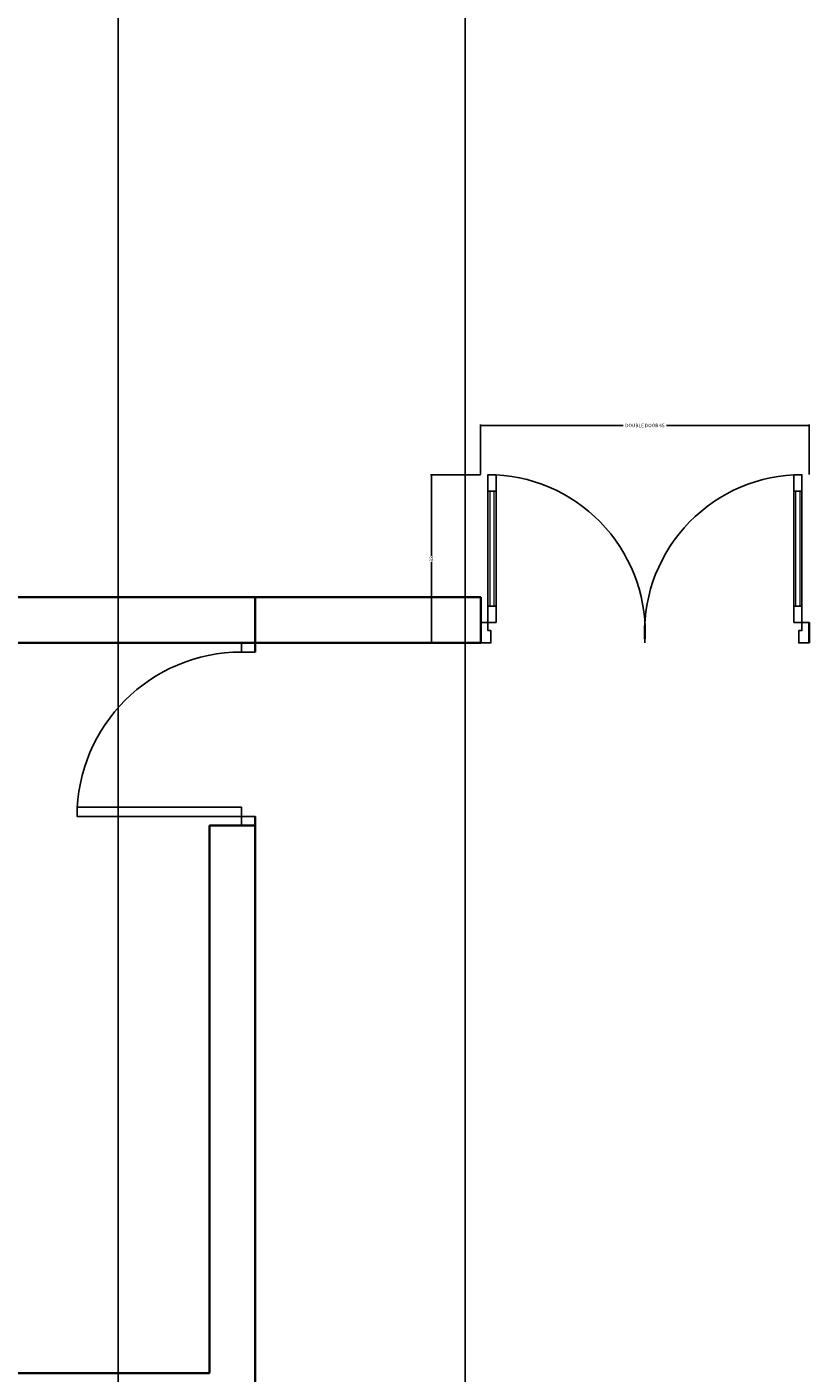
# Model space of a CAD drawing. Units: inches. Extents: x 867 to 1667, y -234 to 788.
# Tile 23 of 42: x 1212 to 1366, y -8 to 258. Entities that reach past the tile are written whole.
import ezdxf

# ---------------------------------------------------------------- set-up
doc = ezdxf.new("R2010")
doc.units = ezdxf.units.IN
doc.header["$MEASUREMENT"] = 0
for name, color, linetype, lineweight in [('A-ANNO-DIMS', 2, 'Continuous', 18), ('A-Door', 150, 'Continuous', 25), ('A-Glaz', 92, 'Continuous', 18), ('A-Wall', 7, 'Continuous', 35)]:
    doc.layers.add(name, color=color, linetype=linetype, lineweight=lineweight)
doc.layers.add('NET 01', color=8, linetype='Continuous')
doc.layers.add('NT', color=1, linetype='Continuous')
doc.styles.get("Standard").update_dxf_attribs({"font": 'arial.ttf'})
doc.dimstyles.get("Standard").update_dxf_attribs({"dimtxt": 0.6875, "dimasz": 0.18, "dimexe": 0.18, "dimexo": 0.0625, "dimgap": 0.09, "dimtad": 0, "dimdec": 4, "dimzin": 0, "dimdsep": 46, "dimlunit": 4, "dimtxsty": 'Standard', "dimcen": 0.09, "dimadec": 0, "dimazin": 0, "dimtfac": 1, "dimtdec": 4, "dimtofl": 0, "dimtmove": 0, "dimatfit": 3, "dimfxl": 1, "dimtolj": 1, "dimtzin": 0, "dimarcsym": 0})

# ---------------------------------------------------------------- blocks, each defined once
blk = doc.blocks.new('A$C292B336C')
at = {"layer": 'A-Door'}
for points in [[(-0.05, 0), (-0.05, 0.9), (0, 0.9), (0, 0)], [(-0.95, 0), (-0.95, -0.075), (-0.9, -0.075), (-0.9, 0)], [(0, 0), (0, -0.075), (0.05, -0.075), (0.05, 0)]]:
    blk.add_lwpolyline(points, close=True, dxfattribs=at)
at = {"layer": 'NET 01'}
blk.add_arc((0, 0), 0.9, 90, 180, dxfattribs=at)
blk = doc.blocks.new('A$C0EE93B68')
at = {"layer": 'A-Door'}
for points in [[(100, 1565), (100, 1600), (0, 1600), (0, 1550), (50, 1550), (60, 1550), (60, 1565)], [(100, 1525), (180, 1525), (180, 1565), (100, 1565)], [(180, 1525), (740, 1525), (740, 1565), (180, 1565)], [(820, 1525), (740, 1525), (740, 1565), (820, 1565)], [(100, 75), (180, 75), (180, 35), (100, 35)], [(180, 75), (740, 75), (740, 35), (180, 35)], [(820, 75), (740, 75), (740, 35), (820, 35)], [(100, 35), (100, 0), (0, 0), (0, 50), (50, 50), (60, 50), (60, 35)]]:
    blk.add_lwpolyline(points, close=True, dxfattribs=at)
at = {"layer": 'A-Glaz'}
for points in [[(180, 1535), (740, 1535), (740, 1555), (180, 1555)], [(180, 65), (740, 65), (740, 45), (180, 45)]]:
    blk.add_lwpolyline(points, close=True, dxfattribs=at)
at = {"layer": 'A-Wall'}
for p, q in [((0, 1600), (100, 1600)), ((0, 0), (100, 0))]:
    blk.add_line(p, q, dxfattribs=at)
at = {"layer": 'NT'}
for centre, start, end in [((51.6, 1567.9), 266.1547, 356.80808), ((51.6, 32.1), 3.19192, 93.8453)]:
    blk.add_arc(centre, 769.6, start, end, dxfattribs=at)
blk = doc.blocks.new('*D11')
at = {"layer": 'A-ANNO-DIMS', "color": 0, "lineweight": -2, "transparency": 16777216}
for p, q in [((1301.35, 169.36), (1301.35, 179.19)), ((1301.53, 179.01), (1329.48, 179.01)), ((1365.93, 179.01), (1337.98, 179.01)), ((1366.11, 169.36), (1366.11, 179.19))]:
    blk.add_line(p, q, dxfattribs=at)
at = {"layer": 'A-ANNO-DIMS', "color": 0, "transparency": 16777216}
for points in [[(1301.53, 179.04), (1301.53, 178.98), (1301.35, 179.01)], [(1365.93, 179.04), (1365.93, 178.98), (1366.11, 179.01)]]:
    blk.add_solid(points, dxfattribs=at)
at = {"layer": 'Defpoints', "color": 0, "transparency": 16777216}
for p in [(1366.11, 179.01), (1301.35, 169.3), (1366.11, 169.3)]:
    blk.add_point(p, dxfattribs=at)
at = {"layer": 'A-ANNO-DIMS', "color": 0, "transparency": 16777216, "insert": (1333.73, 179.01), "char_height": 0.6875, "attachment_point": 5}
blk.add_mtext('\\A1;DOUBLE DOOR 65', dxfattribs=at)
blk = doc.blocks.new('*D12')
at = {"layer": 'A-ANNO-DIMS', "color": 0, "lineweight": -2, "transparency": 16777216}
for p, q in [((1301.29, 169.3), (1291.46, 169.3)), ((1291.64, 169.12), (1291.64, 153.29)), ((1291.64, 136.3), (1291.64, 152.13)), ((1301.29, 136.12), (1291.46, 136.12))]:
    blk.add_line(p, q, dxfattribs=at)
at = {"layer": 'A-ANNO-DIMS', "color": 0, "transparency": 16777216}
for points in [[(1291.61, 169.12), (1291.67, 169.12), (1291.64, 169.3)], [(1291.61, 136.3), (1291.67, 136.3), (1291.64, 136.12)]]:
    blk.add_solid(points, dxfattribs=at)
at = {"layer": 'Defpoints', "color": 0, "transparency": 16777216}
for p in [(1291.64, 169.3), (1301.35, 169.3), (1301.35, 136.12)]:
    blk.add_point(p, dxfattribs=at)
at = {"layer": 'A-ANNO-DIMS', "color": 0, "transparency": 16777216, "insert": (1291.64, 152.71), "char_height": 0.688, "attachment_point": 5, "rotation": 90}
blk.add_mtext('\\A1;33', dxfattribs=at)
blk = doc.blocks.new('*D30')
at = {"layer": 'A-ANNO-DIMS', "color": 0, "lineweight": -2, "transparency": 16777216}
for p, q in [((1229.89, 623.55), (1229.89, -233.54)), ((1298.3, 623.55), (1298.3, -233.54)), ((1230.07, -233.36), (1262.91, -233.36)), ((1298.12, -233.36), (1265.28, -233.36))]:
    blk.add_line(p, q, dxfattribs=at)
at = {"layer": 'A-ANNO-DIMS', "color": 0, "transparency": 16777216}
for points in [[(1230.07, -233.33), (1230.07, -233.39), (1229.89, -233.36)], [(1298.12, -233.33), (1298.12, -233.39), (1298.3, -233.36)]]:
    blk.add_solid(points, dxfattribs=at)
at = {"layer": 'Defpoints', "color": 0, "transparency": 16777216}
for p in [(1229.89, 623.62), (1298.3, 623.62), (1298.3, -233.36)]:
    blk.add_point(p, dxfattribs=at)
at = {"layer": 'A-ANNO-DIMS', "color": 0, "transparency": 16777216, "insert": (1264.09, -233.36), "char_height": 0.688, "attachment_point": 5}
blk.add_mtext('\\A1;68.41', dxfattribs=at)

msp = doc.modelspace()

# ---------------------------------------------------------------- linework, layer by layer
at = {"layer": 'A-Wall'}
for p, q in [((1301.3542, 145.117), (1070.8866, 145.117)), ((1256.8866, 145.117), (1256.8866, 134.3165)), ((1301.3542, 145.117), (1301.3542, 136.117)), ((1301.3542, 136.117), (1070.8866, 136.117)), ((1256.8866, 101.9059), (1256.8866, -16.883)), ((1256.8866, 100.1053), (1247.8866, 100.1053)), ((1247.8866, 100.1053), (1247.8866, -7.883)), ((1247.8866, -7.883), (1079.8866, -7.883))]:
    msp.add_line(p, q, dxfattribs=at)

# ---------------------------------------------------------------- block references
at = {"layer": 'A-Door'}
for name, p, xscale, yscale, zscale, rotation in [('A$C0EE93B68', (1301.3542, 136.117), -0.0404693295706767, 0.0404693295706767, 0.0404693295706767, 270), ('A$C292B336C', (1254.1857, 101.9059), -36.01171521992244, 36.01171521992244, 36.01171521992244, 90)]:
    msp.add_blockref(name, p, dxfattribs=dict(at, xscale=xscale, yscale=yscale, zscale=zscale, rotation=rotation))

# ---------------------------------------------------------------- dimensions: what is measured, and where the dimension line sits
at = {"layer": 'A-ANNO-DIMS'}
dim = msp.add_linear_dim(base=(1298.2966, -233.3581), p1=(1229.8866, 623.617), p2=(1298.2966, 623.617), dimstyle='Standard', override={"dimdec": 2, "dimlfac": 1, "dimrnd": 0, "dimzin": 0, "dimdsep": 46, "dimlunit": 2}, dxfattribs=at)
dim.commit()
dim.dimension.update_dxf_attribs({"geometry": '*D30', "text_midpoint": (1264.0916, -233.3581)})
dim = msp.add_linear_dim(base=(1366.1051, 179.0145), p1=(1301.3542, 169.3019), p2=(1366.1051, 169.3019), text='DOUBLE DOOR <>', dimstyle='Standard', override={"dimdec": 0, "dimlfac": 1, "dimrnd": 0, "dimzin": 0, "dimdsep": 46, "dimlunit": 2}, dxfattribs=at)
dim.commit()
dim.dimension.update_dxf_attribs({"geometry": '*D11', "text_midpoint": (1333.7297, 179.0145)})
dim = msp.add_linear_dim(base=(1291.6416, 169.3019), p1=(1301.3542, 136.117), p2=(1301.3542, 169.3019), angle=90, dimstyle='Standard', override={"dimdec": 0, "dimlfac": 1, "dimrnd": 0, "dimzin": 0, "dimdsep": 46, "dimlunit": 2}, dxfattribs=at)
dim.commit()
dim.dimension.update_dxf_attribs({"geometry": '*D12', "text_midpoint": (1291.6416, 152.7095)})

doc.saveas('drawing.dxf')
